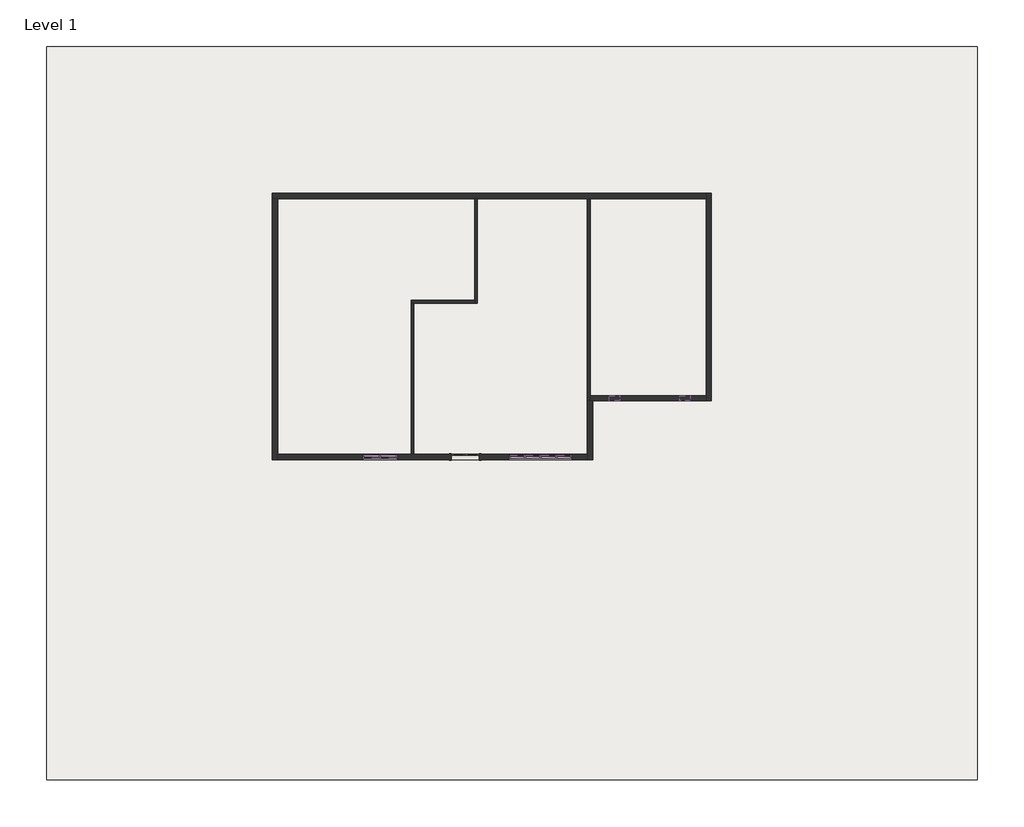
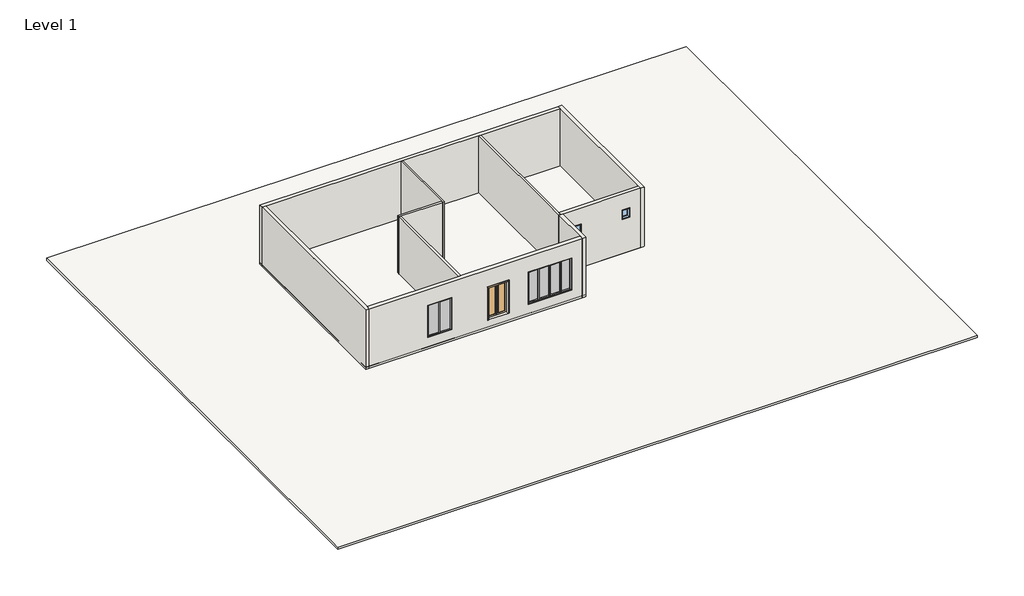
# One storey, incomplete: 20 members, 10 walls, 6 plates, 2 slabs, 2 windows, 1 door.
"""IFC4 building model written with IfcOpenShell, lengths in millimetres."""

from ifc_helpers import new_model, si_unit, frame, origin, origin_with_axes, place, context, project, spatial, polyline, outline, extrude, faceted_brep, transform, mapped, element, save
from components import door_double_glass_4_x_7_21e1f937, member_e5d39754, member_081e0693, member_c33c434a, member_3374d9b6, member_7cbddb58, system_panel_glazed_29c37de9, system_panel_glazed_a68fd5c2, system_panel_glazed_550f7026, fixed_1_x1_542de505

model = new_model("IFC4")

# Units and contexts
model_context = context("Model", 3, world=origin())
ifc_project = project(units=[si_unit("LENGTHUNIT", "METRE", prefix="MILLI")], contexts=[model_context])

# Site, building, storey
site = spatial("IfcSite", under=ifc_project)
building = spatial("IfcBuilding", under=site)
storey = spatial("IfcBuildingStorey", under=building, Name="Level 1", Elevation=0.0)

# Door
placement = place(None, origin())
door_double_glass_4_x_7_shape = door_double_glass_4_x_7_21e1f937(model_context)
element("IfcDoor", 1, ObjectType="Door-Double-Glass : 4' x 7'", at=placement, inside=storey, context=model_context, shape_type="MappedRepresentation", body=[
    mapped(door_double_glass_4_x_7_shape, transform((-1827.2852284, -2816.9185169, 609.6), x_axis=(1.0, 0.0, 0.0), y_axis=(0.0, 1.0, 0.0), z_axis=(0.0, 0.0, 1.0))),
])

# Members
member_shape = member_e5d39754(model_context)
element("IfcMember", 2, ObjectType="Rectangular Mullion : 2.5\" x 5\" rectangular", at=placement, inside=storey, context=model_context, shape_type="MappedRepresentation", body=[
    mapped(member_shape, transform((2738.3647716, -2814.5372669, 2895.6), x_axis=(0.0, 0.0, 1.0), y_axis=(0.0, -1.0, 0.0), z_axis=(1.0, 0.0, 0.0))),
])
element("IfcMember", 3, ObjectType="Rectangular Mullion : 2.5\" x 5\" rectangular", at=placement, inside=storey, context=model_context, shape_type="MappedRepresentation", body=[
    mapped(member_shape, transform((712.7147716, -2814.5372669, 2895.6), x_axis=(0.0, 0.0, 1.0), y_axis=(0.0, -1.0, 0.0), z_axis=(1.0, 0.0, 0.0))),
])
element("IfcMember", 4, ObjectType="Rectangular Mullion : 2.5\" x 5\" rectangular", at=placement, inside=storey, context=model_context, shape_type="MappedRepresentation", body=[
    mapped(member_shape, transform((122.1647716, -2814.5372669, 762.0), x_axis=(0.0, 0.0, -1.0), y_axis=(0.0, -1.0, 0.0), z_axis=(-1.0, 0.0, 0.0))),
])
element("IfcMember", 5, ObjectType="Rectangular Mullion : 2.5\" x 5\" rectangular", at=placement, inside=storey, context=model_context, shape_type="MappedRepresentation", body=[
    mapped(member_shape, transform((2147.8147716, -2814.5372669, 762.0), x_axis=(0.0, 0.0, -1.0), y_axis=(0.0, -1.0, 0.0), z_axis=(-1.0, 0.0, 0.0))),
])
member_2_shape = member_081e0693(model_context)
element("IfcMember", 6, ObjectType="Rectangular Mullion : 2.5\" x 5\" rectangular", at=placement, inside=storey, context=model_context, shape_type="MappedRepresentation", body=[
    mapped(member_2_shape, transform((776.2147716, -2814.5372669, 762.0), x_axis=(0.0, 0.0, -1.0), y_axis=(0.0, -1.0, 0.0), z_axis=(-1.0, 0.0, 0.0))),
])
element("IfcMember", 7, ObjectType="Rectangular Mullion : 2.5\" x 5\" rectangular", at=placement, inside=storey, context=model_context, shape_type="MappedRepresentation", body=[
    mapped(member_2_shape, transform((1462.0147716, -2814.5372669, 762.0), x_axis=(0.0, 0.0, -1.0), y_axis=(0.0, -1.0, 0.0), z_axis=(-1.0, 0.0, 0.0))),
])
element("IfcMember", 8, ObjectType="Rectangular Mullion : 2.5\" x 5\" rectangular", at=placement, inside=storey, context=model_context, shape_type="MappedRepresentation", body=[
    mapped(member_2_shape, transform((1398.5147716, -2814.5372669, 2895.6), x_axis=(0.0, 0.0, 1.0), y_axis=(0.0, -1.0, 0.0), z_axis=(1.0, 0.0, 0.0))),
])
element("IfcMember", 9, ObjectType="Rectangular Mullion : 2.5\" x 5\" rectangular", at=placement, inside=storey, context=model_context, shape_type="MappedRepresentation", body=[
    mapped(member_2_shape, transform((2084.3147716, -2814.5372669, 2895.6), x_axis=(0.0, 0.0, 1.0), y_axis=(0.0, -1.0, 0.0), z_axis=(1.0, 0.0, 0.0))),
])
member_3_shape = member_c33c434a(model_context)
element("IfcMember", 10, ObjectType="Rectangular Mullion : 2.5\" x 5\" rectangular", at=placement, inside=storey, context=model_context, shape_type="MappedRepresentation", body=[
    mapped(member_3_shape, transform((-6208.7852284, -2814.5372669, 2895.6), x_axis=(0.0, 0.0, 1.0), y_axis=(0.0, 1.0, 0.0), z_axis=(-1.0, 0.0, 0.0))),
])
element("IfcMember", 11, ObjectType="Rectangular Mullion : 2.5\" x 5\" rectangular", at=placement, inside=storey, context=model_context, shape_type="MappedRepresentation", body=[
    mapped(member_3_shape, transform((-5478.5352284, -2814.5372669, 2895.6), x_axis=(0.0, 0.0, 1.0), y_axis=(0.0, 1.0, 0.0), z_axis=(-1.0, 0.0, 0.0))),
])
element("IfcMember", 12, ObjectType="Rectangular Mullion : 2.5\" x 5\" rectangular", at=placement, inside=storey, context=model_context, shape_type="MappedRepresentation", body=[
    mapped(member_3_shape, transform((-4811.7852284, -2814.5372669, 762.0), x_axis=(0.0, 0.0, -1.0), y_axis=(0.0, 1.0, 0.0), z_axis=(1.0, 0.0, 0.0))),
])
element("IfcMember", 13, ObjectType="Rectangular Mullion : 2.5\" x 5\" rectangular", at=placement, inside=storey, context=model_context, shape_type="MappedRepresentation", body=[
    mapped(member_3_shape, transform((-5542.0352284, -2814.5372669, 762.0), x_axis=(0.0, 0.0, -1.0), y_axis=(0.0, 1.0, 0.0), z_axis=(1.0, 0.0, 0.0))),
])
member_4_shape = member_3374d9b6(model_context)
element("IfcMember", 14, ObjectType="Rectangular Mullion : 2.5\" x 5\" rectangular", at=placement, inside=storey, context=model_context, shape_type="MappedRepresentation", body=[
    mapped(member_4_shape, transform((58.6647716, -2814.5372669, 2895.6), x_axis=(-1.0, 0.0, 0.0), y_axis=(0.0, -1.0, 0.0), z_axis=(0.0, 0.0, 1.0))),
])
element("IfcMember", 15, ObjectType="Rectangular Mullion : 2.5\" x 5\" rectangular", at=placement, inside=storey, context=model_context, shape_type="MappedRepresentation", body=[
    mapped(member_4_shape, transform((-4748.2852284, -2814.5372669, 2895.6), x_axis=(1.0, 0.0, 0.0), y_axis=(0.0, 1.0, 0.0), z_axis=(0.0, 0.0, 1.0))),
])
element("IfcMember", 16, ObjectType="Rectangular Mullion : 2.5\" x 5\" rectangular", at=placement, inside=storey, context=model_context, shape_type="MappedRepresentation", body=[
    mapped(member_4_shape, transform((2801.8647716, -2814.5372669, 762.0), x_axis=(1.0, 0.0, 0.0), y_axis=(0.0, -1.0, 0.0), z_axis=(0.0, 0.0, -1.0))),
])
element("IfcMember", 17, ObjectType="Rectangular Mullion : 2.5\" x 5\" rectangular", at=placement, inside=storey, context=model_context, shape_type="MappedRepresentation", body=[
    mapped(member_4_shape, transform((-6272.2852284, -2814.5372669, 762.0), x_axis=(-1.0, 0.0, 0.0), y_axis=(0.0, 1.0, 0.0), z_axis=(0.0, 0.0, -1.0))),
])
member_5_shape = member_7cbddb58(model_context)
element("IfcMember", 18, ObjectType="Rectangular Mullion : 2.5\" x 5\" rectangular", at=placement, inside=storey, context=model_context, shape_type="MappedRepresentation", body=[
    mapped(member_5_shape, transform((744.4647716, -2814.5372669, 762.0), x_axis=(1.0, 0.0, 0.0), y_axis=(0.0, -1.0, 0.0), z_axis=(0.0, 0.0, -1.0))),
])
element("IfcMember", 19, ObjectType="Rectangular Mullion : 2.5\" x 5\" rectangular", at=placement, inside=storey, context=model_context, shape_type="MappedRepresentation", body=[
    mapped(member_5_shape, transform((1430.2647716, -2814.5372669, 762.0), x_axis=(1.0, 0.0, 0.0), y_axis=(0.0, -1.0, 0.0), z_axis=(0.0, 0.0, -1.0))),
])
element("IfcMember", 20, ObjectType="Rectangular Mullion : 2.5\" x 5\" rectangular", at=placement, inside=storey, context=model_context, shape_type="MappedRepresentation", body=[
    mapped(member_5_shape, transform((2116.0647716, -2814.5372669, 762.0), x_axis=(1.0, 0.0, 0.0), y_axis=(0.0, -1.0, 0.0), z_axis=(0.0, 0.0, -1.0))),
])
element("IfcMember", 21, ObjectType="Rectangular Mullion : 2.5\" x 5\" rectangular", at=placement, inside=storey, context=model_context, shape_type="MappedRepresentation", body=[
    mapped(member_5_shape, transform((-5510.2852284, -2814.5372669, 762.0), x_axis=(-1.0, 0.0, 0.0), y_axis=(0.0, 1.0, 0.0), z_axis=(0.0, 0.0, -1.0))),
])

# Plates
system_panel_glazed_shape = system_panel_glazed_29c37de9(model_context)
element("IfcPlate", 22, ObjectType="System Panel : Glazed", at=placement, inside=storey, context=model_context, shape_type="MappedRepresentation", body=[
    mapped(system_panel_glazed_shape, transform((417.4397716, -2814.5372669, 825.5), x_axis=(1.0, 0.0, 0.0), y_axis=(0.0, 1.0, 0.0), z_axis=(0.0, 0.0, 1.0))),
])
element("IfcPlate", 23, ObjectType="System Panel : Glazed", at=placement, inside=storey, context=model_context, shape_type="MappedRepresentation", body=[
    mapped(system_panel_glazed_shape, transform((2443.0897716, -2814.5372669, 825.5), x_axis=(1.0, 0.0, 0.0), y_axis=(0.0, 1.0, 0.0), z_axis=(0.0, 0.0, 1.0))),
])
system_panel_glazed_2_shape = system_panel_glazed_a68fd5c2(model_context)
element("IfcPlate", 24, ObjectType="System Panel : Glazed", at=placement, inside=storey, context=model_context, shape_type="MappedRepresentation", body=[
    mapped(system_panel_glazed_2_shape, transform((-5145.1602284, -2814.5372669, 825.5), x_axis=(-1.0, 0.0, 0.0), y_axis=(0.0, -1.0, 0.0), z_axis=(0.0, 0.0, 1.0))),
])
element("IfcPlate", 25, ObjectType="System Panel : Glazed", at=placement, inside=storey, context=model_context, shape_type="MappedRepresentation", body=[
    mapped(system_panel_glazed_2_shape, transform((-5875.4102284, -2814.5372669, 825.5), x_axis=(-1.0, 0.0, 0.0), y_axis=(0.0, -1.0, 0.0), z_axis=(0.0, 0.0, 1.0))),
])
system_panel_glazed_3_shape = system_panel_glazed_550f7026(model_context)
element("IfcPlate", 26, ObjectType="System Panel : Glazed", at=placement, inside=storey, context=model_context, shape_type="MappedRepresentation", body=[
    mapped(system_panel_glazed_3_shape, transform((1087.3647716, -2814.5372669, 825.5), x_axis=(1.0, 0.0, 0.0), y_axis=(0.0, 1.0, 0.0), z_axis=(0.0, 0.0, 1.0))),
])
element("IfcPlate", 27, ObjectType="System Panel : Glazed", at=placement, inside=storey, context=model_context, shape_type="MappedRepresentation", body=[
    mapped(system_panel_glazed_3_shape, transform((1773.1647716, -2814.5372669, 825.5), x_axis=(1.0, 0.0, 0.0), y_axis=(0.0, 1.0, 0.0), z_axis=(0.0, 0.0, 1.0))),
])

# Slabs
element("IfcSlab", 28, ObjectType="6\" floor", at=placement, inside=storey, context=model_context, shape_type="SweptSolid", body=[
    extrude(outline(polyline([(-10171.1852284, -2928.8372669), (-10171.1852284, 8577.3627331), (8802.6147716, 8577.3627331), (8802.6147716, -388.8372669), (3678.1647716, -388.8372669), (3678.1647716, -2928.8372669), (-10171.1852284, -2928.8372669)])), origin_with_axes(), (0.0, 0.0, 1.0), 152.4),
])
element("IfcSlab", 29, ObjectType="6\" floor 2", at=placement, inside=storey, context=model_context, shape_type="SweptSolid", body=[
    extrude(outline(polyline([(20305.2083938, 14922.2756503), (20305.2083938, -16776.9243497), (-19928.3916062, -16776.9243497), (-19928.3916062, 14922.2756503), (20305.2083938, 14922.2756503)])), frame((0.0, 0.0, -152.4), z_axis=(0.0, 0.0, 1.0), x_axis=(1.0, 0.0, 0.0)), (0.0, 0.0, 1.0), 152.4),
])

# Walls
element("IfcWall", 30, ObjectType="4.5\" wall", at=placement, inside=storey, context=model_context, shape_type="Brep", body=[
    faceted_brep([(3449.5647716, 8348.7627331, 0.0), (3449.5647716, -388.8372669, 0.0), (3449.5647716, -388.8372669, 3962.4), (3449.5647716, 8348.7627331, 3962.4), (3563.8647716, 8348.7627331, 0.0), (3563.8647716, 8348.7627331, 3962.4), (3563.8647716, -160.2372669, 3962.4), (3563.8647716, -388.8372669, 3962.4), (3563.8647716, -388.8372669, 0.0), (3563.8647716, -160.2372669, 0.0)], [[[0, 1, 2, 3]], [[4, 5, 6, 7, 8, 9]], [[1, 0, 4, 9, 8]], [[0, 3, 5, 4]], [[2, 1, 8, 7]], [[3, 2, 7, 6, 5]]]),
])
element("IfcWall", 31, ObjectType="4.5\" wall", at=placement, inside=storey, context=model_context, shape_type="Brep", body=[
    faceted_brep([(-1427.2352284, 8348.7627331, 0.0), (-1427.2352284, 3948.2127331, 0.0), (-1427.2352284, 3833.9127331, 0.0), (-1427.2352284, 3833.9127331, 3962.4), (-1427.2352284, 3948.2127331, 3962.4), (-1427.2352284, 8348.7627331, 3962.4), (-1312.9352284, 8348.7627331, 0.0), (-1312.9352284, 8348.7627331, 3962.4), (-1312.9352284, 3833.9127331, 3962.4), (-1312.9352284, 3833.9127331, 0.0)], [[[0, 1, 2, 3, 4, 5]], [[6, 7, 8, 9]], [[2, 1, 0, 6, 9]], [[0, 5, 7, 6]], [[3, 2, 9, 8]], [[5, 4, 3, 8, 7]]]),
])
element("IfcWall", 32, ObjectType="4.5\" wall", at=placement, inside=storey, context=model_context, shape_type="Brep", body=[
    faceted_brep([(-1427.2352284, 3948.2127331, 0.0), (-4170.4352284, 3948.2127331, 0.0), (-4170.4352284, 3948.2127331, 3962.4), (-1427.2352284, 3948.2127331, 3962.4), (-1427.2352284, 3833.9127331, 0.0), (-1427.2352284, 3833.9127331, 3962.4), (-4056.1352284, 3833.9127331, 3962.4), (-4170.4352284, 3833.9127331, 3962.4), (-4170.4352284, 3833.9127331, 0.0), (-4056.1352284, 3833.9127331, 0.0)], [[[0, 1, 2, 3]], [[4, 5, 6, 7, 8, 9]], [[1, 0, 4, 9, 8]], [[0, 3, 5, 4]], [[2, 1, 8, 7]], [[3, 2, 7, 6, 5]]]),
])
element("IfcWall", 33, ObjectType="4.5\" wall", at=placement, inside=storey, context=model_context, shape_type="SweptSolid", body=[
    extrude(outline(polyline([(-4170.4352284, -2700.2372669), (-4170.4352284, 3833.9127331), (-4056.1352284, 3833.9127331), (-4056.1352284, -2700.2372669), (-4170.4352284, -2700.2372669)])), origin_with_axes(), (0.0, 0.0, 1.0), 3962.4),
])
element("IfcWall", 34, ObjectType="9\" wall", at=placement, inside=storey, context=model_context, shape_type="Brep", body=[
    faceted_brep([(-10171.1852284, 8348.7627331, 0.0), (-9942.5852284, 8348.7627331, 0.0), (-1427.2352284, 8348.7627331, 0.0), (-1312.9352284, 8348.7627331, 0.0), (3449.5647716, 8348.7627331, 0.0), (3563.8647716, 8348.7627331, 0.0), (8574.0147716, 8348.7627331, 0.0), (8574.0147716, 8348.7627331, 3962.4), (3563.8647716, 8348.7627331, 3962.4), (3449.5647716, 8348.7627331, 3962.4), (-1312.9352284, 8348.7627331, 3962.4), (-1427.2352284, 8348.7627331, 3962.4), (-9942.5852284, 8348.7627331, 3962.4), (-10171.1852284, 8348.7627331, 3962.4), (-10171.1852284, 8577.3627331, 0.0), (-10171.1852284, 8577.3627331, 3962.4), (8574.0147716, 8577.3627331, 3962.4), (8574.0147716, 8577.3627331, 0.0)], [[[0, 1, 2, 3, 4, 5, 6, 7, 8, 9, 10, 11, 12, 13]], [[14, 15, 16, 17]], [[6, 5, 4, 3, 2, 1, 0, 14, 17]], [[0, 13, 15, 14]], [[7, 6, 17, 16]], [[13, 12, 11, 10, 9, 8, 7, 16, 15]]]),
])
element("IfcWall", 35, ObjectType="9\" wall", at=placement, inside=storey, context=model_context, shape_type="Brep", body=[
    faceted_brep([(-9942.5852284, -2928.8372669, 0.0), (-9942.5852284, -2700.2372669, 0.0), (-9942.5852284, 8348.7627331, 0.0), (-9942.5852284, 8348.7627331, 3962.4), (-9942.5852284, -2700.2372669, 3962.4), (-9942.5852284, -2928.8372669, 3962.4), (-10171.1852284, -2928.8372669, 0.0), (-10171.1852284, -2928.8372669, 3962.4), (-10171.1852284, 8348.7627331, 3962.4), (-10171.1852284, 8348.7627331, 0.0)], [[[0, 1, 2, 3, 4, 5]], [[6, 7, 8, 9]], [[2, 1, 0, 6, 9]], [[0, 5, 7, 6]], [[3, 2, 9, 8]], [[5, 4, 3, 8, 7]]]),
])
element("IfcWall", 36, ObjectType="9\" wall", at=placement, inside=storey, context=model_context, shape_type="Brep", body=[
    faceted_brep([(8574.0147716, 8577.3627331, 0.0), (8574.0147716, 8348.7627331, 0.0), (8574.0147716, -160.2372669, 0.0), (8574.0147716, -388.8372669, 0.0), (8574.0147716, -388.8372669, 3962.4), (8574.0147716, -160.2372669, 3962.4), (8574.0147716, 8348.7627331, 3962.4), (8574.0147716, 8577.3627331, 3962.4), (8802.6147716, 8577.3627331, 0.0), (8802.6147716, 8577.3627331, 3962.4), (8802.6147716, -388.8372669, 3962.4), (8802.6147716, -388.8372669, 0.0)], [[[0, 1, 2, 3, 4, 5, 6, 7]], [[8, 9, 10, 11]], [[3, 2, 1, 0, 8, 11]], [[0, 7, 9, 8]], [[7, 6, 5, 4, 10, 9]], [[4, 3, 11, 10]]]),
])
element("IfcWall", 37, ObjectType="9\" wall", at=placement, inside=storey, context=model_context, shape_type="Brep", body=[
    faceted_brep([(8574.0147716, -160.2372669, 0.0), (3563.8647716, -160.2372669, 0.0), (3563.8647716, -160.2372669, 3962.4), (8574.0147716, -160.2372669, 3962.4), (7900.9147716, -160.2372669, 2895.6), (7443.7147716, -160.2372669, 2895.6), (7443.7147716, -160.2372669, 2286.0), (7900.9147716, -160.2372669, 2286.0), (4395.7147716, -160.2372669, 2895.6), (4395.7147716, -160.2372669, 2286.0), (4852.9147716, -160.2372669, 2286.0), (4852.9147716, -160.2372669, 2895.6), (8574.0147716, -388.8372669, 0.0), (8574.0147716, -388.8372669, 3962.4), (3678.1647716, -388.8372669, 3962.4), (3563.8647716, -388.8372669, 3962.4), (3563.8647716, -388.8372669, 0.0), (3678.1647716, -388.8372669, 0.0), (7900.9147716, -388.8372669, 2895.6), (7900.9147716, -388.8372669, 2286.0), (7443.7147716, -388.8372669, 2286.0), (7443.7147716, -388.8372669, 2895.6), (4395.7147716, -388.8372669, 2895.6), (4852.9147716, -388.8372669, 2895.6), (4852.9147716, -388.8372669, 2286.0), (4395.7147716, -388.8372669, 2286.0)], [[[0, 1, 2, 3], [4, 5, 6, 7], [8, 9, 10, 11]], [[12, 13, 14, 15, 16, 17], [18, 19, 20, 21], [22, 23, 24, 25]], [[1, 0, 12, 17, 16]], [[2, 1, 16, 15]], [[3, 2, 15, 14, 13]], [[19, 18, 4, 7]], [[20, 19, 7, 6]], [[21, 20, 6, 5]], [[18, 21, 5, 4]], [[9, 8, 22, 25]], [[10, 9, 25, 24]], [[11, 10, 24, 23]], [[8, 11, 23, 22]], [[0, 3, 13, 12]]]),
])
element("IfcWall", 38, ObjectType="9\" wall", at=placement, inside=storey, context=model_context, shape_type="Brep", body=[
    faceted_brep([(3449.5647716, -388.8372669, 0.0), (3449.5647716, -2700.2372669, 0.0), (3449.5647716, -2928.8372669, 0.0), (3449.5647716, -2928.8372669, 3962.4), (3449.5647716, -2700.2372669, 3962.4), (3449.5647716, -388.8372669, 3962.4), (3678.1647716, -388.8372669, 0.0), (3678.1647716, -388.8372669, 3962.4), (3678.1647716, -2928.8372669, 3962.4), (3678.1647716, -2928.8372669, 0.0), (3563.8647716, -388.8372669, 0.0), (3563.8647716, -388.8372669, 3962.4)], [[[0, 1, 2, 3, 4, 5]], [[6, 7, 8, 9]], [[2, 1, 0, 10, 6, 9]], [[0, 5, 11, 7, 6, 10]], [[3, 2, 9, 8]], [[5, 4, 3, 8, 7, 11]]]),
])
element("IfcWall", 39, ObjectType="9\" wall", at=placement, inside=storey, context=model_context, shape_type="Brep", body=[
    faceted_brep([(3449.5647716, -2700.2372669, 0.0), (-4056.1352284, -2700.2372669, 0.0), (-4170.4352284, -2700.2372669, 0.0), (-9942.5852284, -2700.2372669, 0.0), (-9942.5852284, -2700.2372669, 3962.4), (-4170.4352284, -2700.2372669, 3962.4), (-4056.1352284, -2700.2372669, 3962.4), (3449.5647716, -2700.2372669, 3962.4), (-2436.8852284, -2700.2372669, 609.6), (-1217.6852284, -2700.2372669, 609.6), (-1217.6852284, -2700.2372669, 2743.2), (-2436.8852284, -2700.2372669, 2743.2), (58.6647716, -2700.2372669, 2895.6), (58.6647716, -2700.2372669, 762.0), (2801.8647716, -2700.2372669, 762.0), (2801.8647716, -2700.2372669, 2895.6), (-4748.2852284, -2700.2372669, 762.0), (-4748.2852284, -2700.2372669, 2895.6), (-6272.2852284, -2700.2372669, 2895.6), (-6272.2852284, -2700.2372669, 762.0), (-9942.5852284, -2928.8372669, 0.0), (3449.5647716, -2928.8372669, 0.0), (3449.5647716, -2928.8372669, 3962.4), (-9942.5852284, -2928.8372669, 3962.4), (-2436.8852284, -2928.8372669, 609.6), (-2436.8852284, -2928.8372669, 2743.2), (-1217.6852284, -2928.8372669, 2743.2), (-1217.6852284, -2928.8372669, 609.6), (58.6647716, -2928.8372669, 762.0), (58.6647716, -2928.8372669, 2895.6), (2801.8647716, -2928.8372669, 2895.6), (2801.8647716, -2928.8372669, 762.0), (-4748.2852284, -2928.8372669, 2895.6), (-4748.2852284, -2928.8372669, 762.0), (-6272.2852284, -2928.8372669, 762.0), (-6272.2852284, -2928.8372669, 2895.6)], [[[0, 1, 2, 3, 4, 5, 6, 7], [8, 9, 10, 11], [12, 13, 14, 15], [16, 17, 18, 19]], [[20, 21, 22, 23], [24, 25, 26, 27], [28, 29, 30, 31], [32, 33, 34, 35]], [[3, 2, 1, 0, 21, 20]], [[4, 3, 20, 23]], [[0, 7, 22, 21]], [[9, 8, 24, 27]], [[10, 9, 27, 26]], [[11, 10, 26, 25]], [[8, 11, 25, 24]], [[28, 13, 12, 29]], [[29, 12, 15, 30]], [[30, 15, 14, 31]], [[13, 28, 31, 14]], [[16, 33, 32, 17]], [[17, 32, 35, 18]], [[34, 19, 18, 35]], [[33, 16, 19, 34]], [[7, 6, 5, 4, 23, 22]]]),
])

# Windows
fixed_1_x1_shape = fixed_1_x1_542de505(model_context)
element("IfcWindow", 40, ObjectType="Fixed : 1'x1'", at=placement, inside=storey, context=model_context, shape_type="MappedRepresentation", body=[
    mapped(fixed_1_x1_shape, transform((7710.4147716, -274.5372669, 1981.2), x_axis=(1.0, 0.0, 0.0), y_axis=(0.0, 1.0, 0.0), z_axis=(0.0, 0.0, 1.0))),
])
element("IfcWindow", 41, ObjectType="Fixed : 1'x1'", at=placement, inside=storey, context=model_context, shape_type="MappedRepresentation", body=[
    mapped(fixed_1_x1_shape, transform((4586.2147716, -274.5372669, 1981.2), x_axis=(-1.0, 0.0, 0.0), y_axis=(0.0, -1.0, 0.0), z_axis=(0.0, 0.0, 1.0))),
])

save(model, "model.ifc")

# Revit data of these elements
# Type "Door-Double-Glass : 4' x 7'"
#   Type Mark = "16"
#   Construction Type Id = "opn-d45"
#   Assembly Code = "C1020"
#   Analytic Construction = "Wood frame, double glass door "
#   W = 2' - 0"
#   Thickness = 0' - 2"
#   Thermal Resistance (R) = 1.8150 (h·ft²·°F)/BTU
#   Swing Angle [instance default] = 90.00°
#   Heat Transfer Coefficient (U) = 0.5510 BTU/(h·ft²·°F)
#   Height = 7' - 0"
#   Bottom Rail = 0' - 4"
#   Top Rail = 0' - 4"
#   Stiles = 0' - 4"
#   Trim Projection = 0' - 1"
#   Trim Width = 0' - 3"
#   Width = 4' - 0"
#   Define Thermal Properties by = 1
#   Glazing = Glass
#   Panel Material = door black
#   Trim Material = Paint - Sienna
#   Visual Light Transmittance = 0
#   Solar Heat Gain Coefficient = 0
#   Function = (empty or 0)
#   Wall Closure = (empty or 0)
# Type "Rectangular Mullion : 2.5\" x 5\" rectangular"
#   built-in parameter 1007304 = 0.416667 (stored number, unit not read)
#   built-in parameter 1007301 = 0.104167 (stored number, unit not read)
#   built-in parameter 1007300 = 0.104167 (stored number, unit not read)
# Type "System Panel : Glazed"
#   Construction Type Id = "GSP4R"
#   Analytic Construction = "1/8 in Pilkington single glazing"
#   Visual Light Transmittance = 0.9
#   Solar Heat Gain Coefficient = 0.86
#   Heat Transfer Coefficient (U) = 1.18115 BTU/(h·ft²·°F)
#   Define Thermal Properties by = 1
# Type "6\" floor"
#   Assembly Code = "B1010"
#   Function = 0
#   Layers, outside or top first: 0' - 6" "Wall" (function 1)
# Type "6\" floor 2"
#   Assembly Code = "B1010"
#   Function = 0
#   Layers, outside or top first: 0' - 6" "ground tiles" (function 1)
# Type "4.5\" wall"
#   Assembly Code = "B2010"
#   Layers, outside or top first: 0' - 4 1/2" "Wall" (function 1)
# Type "9\" wall"
#   Assembly Code = "B2010"
#   Layers, outside or top first: 0' - 9" "Wall" (function 1)
# Type "Fixed : 1'x1'"
#   Type Mark = "18"
#   Construction Type Id = "GSP4R"
#   Assembly Code = "B2020100"
#   Analytic Construction = "1/8 in Pilkington single glazing"
#   Visual Light Transmittance = 0.9
#   Solar Heat Gain Coefficient = 0.78
#   Heat Transfer Coefficient (U) = 0.6496 BTU/(h·ft²·°F)
#   Height = 2' - 0"
#   Default Sill Height = 1' - 0"
#   Width = 1' - 6"
#   Window Inset = 0' - 0 3/4"
#   Define Thermal Properties by = 1
#   Glass Pane Material = Glass
#   Sash Material = door black
#   Wall Closure = (empty or 0)
# Element 1 (IfcDoor, "Door-Double-Glass : 4' x 7'")
#   Swing Angle = 90.00°
#   Phase Created = New Construction
#   Materials on its faces: "door black", "Paint - Sienna", "Glass"
# Elements 2, 3, 4, 5, 6, 7, 8, 9, 10, 11, 12, 13, 14, 15, 16, 17, 18, 19, 20, 21 (IfcMember, "Rectangular Mullion : 2.5\" x 5\" rectangular")
#   Phase Created = New Construction
#   Materials on its faces: "door black"
# Elements 22, 23, 24, 25, 26, 27 (IfcPlate, "System Panel : Glazed")
#   Phase Created = New Construction
#   Materials on its faces: "Glass"
# Element 28 (IfcSlab, "6\" floor")
#   built-in parameter 1001955 = -1.5708 (stored number, unit not read)
#   Height Offset From Level = 0' - 6"
#   Phase Created = New Construction
#   Materials on its faces: "Wall"
# Element 29 (IfcSlab, "6\" floor 2")
#   Height Offset From Level = 0' - 0"
#   Phase Created = New Construction
#   Materials on its faces: "ground tiles"
# Elements 30, 31, 32, 33 (IfcWall, "4.5\" wall")
#   Top Offset = 0' - 0"
#   Base Offset = 0' - 0"
#   wall height = 13' - 0"
#   Phase Created = New Construction
#   Base Constraint = Level 1
#   Top Constraint = Level 2
#   Materials on its faces: "Wall"
# Elements 34, 35, 36, 37, 38, 39 (IfcWall, "9\" wall")
#   Top Offset = 0' - 0"
#   Base Offset = 0' - 0"
#   wall height = 13' - 0"
#   Phase Created = New Construction
#   Base Constraint = Level 1
#   Top Constraint = Level 2
#   Materials on its faces: "Wall"
# Element 40 (IfcWindow, "Fixed : 1'x1'")
#   Mark = "1"
#   Phase Created = New Construction
#   Materials on its faces: "door black", "Glass"
# Element 41 (IfcWindow, "Fixed : 1'x1'")
#   Mark = "2"
#   Phase Created = New Construction
#   Materials on its faces: "door black", "Glass"
# Materials
#   "Glass": class "Glass", colour RGB 0 128 192, transparency 0.75, Description = "Soda Lime Glass", Cost = 0
#   "door black": class "Generic", colour RGB 120 120 120, transparency 0, Cost = 0
#   "Paint - Sienna": colour RGB 118 70 51, transparency 0, Cost = 0
#   "Wall": class "Generic", colour RGB 120 120 120, transparency 0, Cost = 0
#   "ground tiles": class "Generic", colour RGB 120 120 120, transparency 0, Cost = 0
